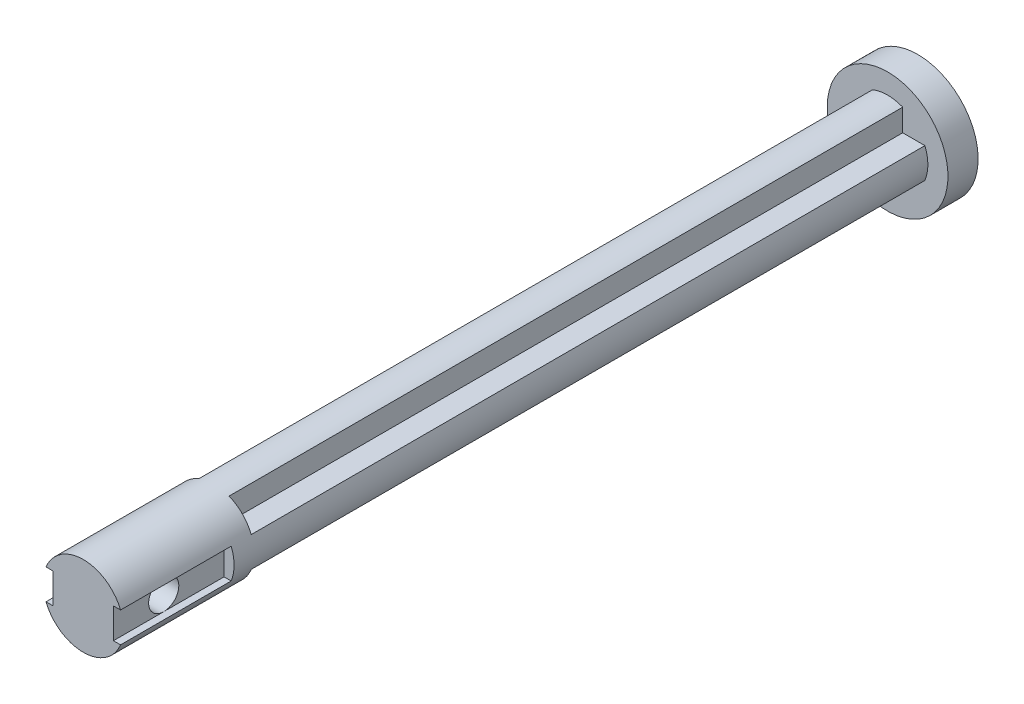
ISO-10303-21;
HEADER;
FILE_DESCRIPTION(('STEP AP214'),'2;1');
FILE_NAME('part.step','',(''),(''),'','','');
FILE_SCHEMA(('AUTOMOTIVE_DESIGN { 1 0 10303 214 1 1 1 1 }'));
ENDSEC;
DATA;
#1=APPLICATION_CONTEXT('core data for automotive mechanical design processes');
#2=APPLICATION_PROTOCOL_DEFINITION('international standard','automotive_design',2000,#1);
#3=PRODUCT_CONTEXT('',#1,'mechanical');
#4=PRODUCT('Part','Part','',(#3));
#5=PRODUCT_RELATED_PRODUCT_CATEGORY('part','',(#4));
#6=PRODUCT_DEFINITION_FORMATION('','',#4);
#7=PRODUCT_DEFINITION_CONTEXT('part definition',#1,'design');
#8=PRODUCT_DEFINITION('design','',#6,#7);
#9=PRODUCT_DEFINITION_SHAPE('','',#8);
#10=(LENGTH_UNIT() NAMED_UNIT(*) SI_UNIT(.MILLI.,.METRE.));
#11=(NAMED_UNIT(*) PLANE_ANGLE_UNIT() SI_UNIT($,.RADIAN.));
#12=(NAMED_UNIT(*) SI_UNIT($,.STERADIAN.) SOLID_ANGLE_UNIT());
#13=UNCERTAINTY_MEASURE_WITH_UNIT(LENGTH_MEASURE(1.E-05),#10,'distance_accuracy_value','');
#14=(GEOMETRIC_REPRESENTATION_CONTEXT(3) GLOBAL_UNCERTAINTY_ASSIGNED_CONTEXT((#13)) GLOBAL_UNIT_ASSIGNED_CONTEXT((#10,
#11,#12)) REPRESENTATION_CONTEXT('',''));
#15=CARTESIAN_POINT('',(0.,0.,0.));
#16=DIRECTION('',(0.,0.,1.));
#17=DIRECTION('',(1.,0.,0.));
#18=AXIS2_PLACEMENT_3D('',#15,#16,#17);
#19=CARTESIAN_POINT('',(3.,0.,69.));
#20=DIRECTION('',(-1.,0.,0.));
#21=DIRECTION('',(0.,0.,1.));
#22=AXIS2_PLACEMENT_3D('',#19,#20,#21);
#23=PLANE('',#22);
#24=CARTESIAN_POINT('',(3.,0.,75.));
#25=DIRECTION('',(1.,0.,0.));
#26=DIRECTION('',(0.,0.,-1.));
#27=AXIS2_PLACEMENT_3D('',#24,#25,#26);
#28=CIRCLE('',#27,1.5);
#29=CARTESIAN_POINT('',(3.,1.5,75.));
#30=VERTEX_POINT('',#29);
#31=CARTESIAN_POINT('',(3.,-1.5,75.));
#32=VERTEX_POINT('',#31);
#33=EDGE_CURVE('E54',#30,#32,#28,.T.);
#34=ORIENTED_EDGE('',*,*,#33,.F.);
#35=DIRECTION('',(0.,0.,1.));
#36=VECTOR('',#35,1.);
#37=CARTESIAN_POINT('',(3.,1.5,69.));
#38=LINE('',#37,#36);
#39=CARTESIAN_POINT('',(3.,1.5,80.));
#40=VERTEX_POINT('',#39);
#41=EDGE_CURVE('E381',#30,#40,#38,.T.);
#42=ORIENTED_EDGE('',*,*,#41,.T.);
#43=DIRECTION('',(0.,-1.,0.));
#44=VECTOR('',#43,1.);
#45=CARTESIAN_POINT('',(3.,0.,80.));
#46=LINE('',#45,#44);
#47=CARTESIAN_POINT('',(3.,-1.5,80.));
#48=VERTEX_POINT('',#47);
#49=EDGE_CURVE('E366',#40,#48,#46,.T.);
#50=ORIENTED_EDGE('',*,*,#49,.T.);
#51=DIRECTION('',(0.,0.,1.));
#52=VECTOR('',#51,1.);
#53=CARTESIAN_POINT('',(3.,-1.5,69.));
#54=LINE('',#53,#52);
#55=EDGE_CURVE('E364',#32,#48,#54,.T.);
#56=ORIENTED_EDGE('',*,*,#55,.F.);
#57=EDGE_LOOP('',(#34,#42,#50,#56));
#58=FACE_BOUND('',#57,.T.);
#59=ADVANCED_FACE('F41',(#58),#23,.F.);
#60=CARTESIAN_POINT('',(-3.,0.,69.));
#61=DIRECTION('',(-1.,0.,0.));
#62=DIRECTION('',(0.,-1.,0.));
#63=AXIS2_PLACEMENT_3D('',#60,#61,#62);
#64=PLANE('',#63);
#65=CARTESIAN_POINT('',(-3.,0.,75.));
#66=DIRECTION('',(-1.,0.,0.));
#67=DIRECTION('',(0.,-1.,0.));
#68=AXIS2_PLACEMENT_3D('',#65,#66,#67);
#69=CIRCLE('',#68,1.5);
#70=CARTESIAN_POINT('',(-3.,-1.5,75.));
#71=VERTEX_POINT('',#70);
#72=CARTESIAN_POINT('',(-3.,1.5,75.));
#73=VERTEX_POINT('',#72);
#74=EDGE_CURVE('E64',#71,#73,#69,.T.);
#75=ORIENTED_EDGE('',*,*,#74,.F.);
#76=DIRECTION('',(0.,0.,1.));
#77=VECTOR('',#76,1.);
#78=CARTESIAN_POINT('',(-3.,-1.5,69.));
#79=LINE('',#78,#77);
#80=CARTESIAN_POINT('',(-3.,-1.5,80.));
#81=VERTEX_POINT('',#80);
#82=EDGE_CURVE('E405',#71,#81,#79,.T.);
#83=ORIENTED_EDGE('',*,*,#82,.T.);
#84=DIRECTION('',(0.,-1.,0.));
#85=VECTOR('',#84,1.);
#86=CARTESIAN_POINT('',(-3.,0.,80.));
#87=LINE('',#86,#85);
#88=CARTESIAN_POINT('',(-3.,1.5,80.));
#89=VERTEX_POINT('',#88);
#90=EDGE_CURVE('E406',#89,#81,#87,.T.);
#91=ORIENTED_EDGE('',*,*,#90,.F.);
#92=DIRECTION('',(0.,0.,1.));
#93=VECTOR('',#92,1.);
#94=CARTESIAN_POINT('',(-3.,1.5,69.));
#95=LINE('',#94,#93);
#96=EDGE_CURVE('E407',#73,#89,#95,.T.);
#97=ORIENTED_EDGE('',*,*,#96,.F.);
#98=EDGE_LOOP('',(#75,#83,#91,#97));
#99=FACE_BOUND('',#98,.T.);
#100=ADVANCED_FACE('F334',(#99),#64,.T.);
#101=CARTESIAN_POINT('',(0.,0.,80.));
#102=DIRECTION('',(0.,0.,1.));
#103=DIRECTION('',(1.,0.,0.));
#104=AXIS2_PLACEMENT_3D('',#101,#102,#103);
#105=PLANE('',#104);
#106=CARTESIAN_POINT('',(0.,0.,80.));
#107=DIRECTION('',(0.,0.,1.));
#108=DIRECTION('',(1.,0.,0.));
#109=AXIS2_PLACEMENT_3D('',#106,#107,#108);
#110=CIRCLE('',#109,4.);
#111=CARTESIAN_POINT('',(3.70809924354783,1.5,80.));
#112=VERTEX_POINT('',#111);
#113=CARTESIAN_POINT('',(-3.70809924354783,1.5,80.));
#114=VERTEX_POINT('',#113);
#115=EDGE_CURVE('E207',#112,#114,#110,.T.);
#116=ORIENTED_EDGE('',*,*,#115,.T.);
#117=DIRECTION('',(1.,0.,0.));
#118=VECTOR('',#117,1.);
#119=CARTESIAN_POINT('',(0.,1.5,80.));
#120=LINE('',#119,#118);
#121=EDGE_CURVE('E382',#114,#89,#120,.T.);
#122=ORIENTED_EDGE('',*,*,#121,.T.);
#123=ORIENTED_EDGE('',*,*,#90,.T.);
#124=DIRECTION('',(1.,0.,0.));
#125=VECTOR('',#124,1.);
#126=CARTESIAN_POINT('',(0.,-1.5,80.));
#127=LINE('',#126,#125);
#128=CARTESIAN_POINT('',(-3.70809924354783,-1.5,80.));
#129=VERTEX_POINT('',#128);
#130=EDGE_CURVE('E415',#129,#81,#127,.T.);
#131=ORIENTED_EDGE('',*,*,#130,.F.);
#132=CARTESIAN_POINT('',(3.70809924354783,-1.5,80.));
#133=VERTEX_POINT('',#132);
#134=EDGE_CURVE('E215',#129,#133,#110,.T.);
#135=ORIENTED_EDGE('',*,*,#134,.T.);
#136=DIRECTION('',(1.,0.,0.));
#137=VECTOR('',#136,1.);
#138=CARTESIAN_POINT('',(0.,-1.5,80.));
#139=LINE('',#138,#137);
#140=EDGE_CURVE('E389',#48,#133,#139,.T.);
#141=ORIENTED_EDGE('',*,*,#140,.F.);
#142=ORIENTED_EDGE('',*,*,#49,.F.);
#143=DIRECTION('',(1.,0.,0.));
#144=VECTOR('',#143,1.);
#145=CARTESIAN_POINT('',(0.,1.5,80.));
#146=LINE('',#145,#144);
#147=EDGE_CURVE('E383',#40,#112,#146,.T.);
#148=ORIENTED_EDGE('',*,*,#147,.T.);
#149=EDGE_LOOP('',(#116,#122,#123,#131,#135,#141,#142,#148));
#150=FACE_BOUND('',#149,.T.);
#151=ADVANCED_FACE('F338',(#150),#105,.T.);
#152=CARTESIAN_POINT('',(0.,1.49999999999998,67.));
#153=DIRECTION('',(0.,1.,0.));
#154=DIRECTION('',(-1.,0.,0.));
#155=AXIS2_PLACEMENT_3D('',#152,#153,#154);
#156=PLANE('',#155);
#157=DIRECTION('',(1.,0.,0.));
#158=VECTOR('',#157,1.);
#159=CARTESIAN_POINT('',(0.,1.49999999999998,0.));
#160=LINE('',#159,#158);
#161=CARTESIAN_POINT('',(-3.70809924354783,1.5,0.));
#162=VERTEX_POINT('',#161);
#163=CARTESIAN_POINT('',(-1.50000000000001,1.49999999999999,0.));
#164=VERTEX_POINT('',#163);
#165=EDGE_CURVE('E191',#162,#164,#160,.T.);
#166=ORIENTED_EDGE('',*,*,#165,.F.);
#167=DIRECTION('',(0.,0.,-1.));
#168=VECTOR('',#167,1.);
#169=CARTESIAN_POINT('',(-3.70809924354783,1.5,67.));
#170=LINE('',#169,#168);
#171=CARTESIAN_POINT('',(-3.70809924354783,1.5,67.));
#172=VERTEX_POINT('',#171);
#173=EDGE_CURVE('E11',#172,#162,#170,.T.);
#174=ORIENTED_EDGE('',*,*,#173,.F.);
#175=DIRECTION('',(1.,0.,0.));
#176=VECTOR('',#175,1.);
#177=CARTESIAN_POINT('',(0.,1.49999999999998,67.));
#178=LINE('',#177,#176);
#179=CARTESIAN_POINT('',(-1.50000000000001,1.49999999999999,67.));
#180=VERTEX_POINT('',#179);
#181=EDGE_CURVE('E242',#172,#180,#178,.T.);
#182=ORIENTED_EDGE('',*,*,#181,.T.);
#183=DIRECTION('',(0.,0.,-1.));
#184=VECTOR('',#183,1.);
#185=CARTESIAN_POINT('',(-1.50000000000001,1.49999999999999,67.));
#186=LINE('',#185,#184);
#187=EDGE_CURVE('E210',#180,#164,#186,.T.);
#188=ORIENTED_EDGE('',*,*,#187,.T.);
#189=EDGE_LOOP('',(#166,#174,#182,#188));
#190=FACE_BOUND('',#189,.T.);
#191=ADVANCED_FACE('F43',(#190),#156,.T.);
#192=CARTESIAN_POINT('',(0.,-1.5,67.));
#193=DIRECTION('',(0.,1.,0.));
#194=DIRECTION('',(-1.,0.,0.));
#195=AXIS2_PLACEMENT_3D('',#192,#193,#194);
#196=PLANE('',#195);
#197=DIRECTION('',(1.,0.,0.));
#198=VECTOR('',#197,1.);
#199=CARTESIAN_POINT('',(0.,-1.5,0.));
#200=LINE('',#199,#198);
#201=CARTESIAN_POINT('',(-3.70809924354783,-1.5,0.));
#202=VERTEX_POINT('',#201);
#203=CARTESIAN_POINT('',(-1.50000000000003,-1.5,0.));
#204=VERTEX_POINT('',#203);
#205=EDGE_CURVE('E192',#202,#204,#200,.T.);
#206=ORIENTED_EDGE('',*,*,#205,.T.);
#207=DIRECTION('',(0.,0.,-1.));
#208=VECTOR('',#207,1.);
#209=CARTESIAN_POINT('',(-1.50000000000003,-1.5,67.));
#210=LINE('',#209,#208);
#211=CARTESIAN_POINT('',(-1.50000000000003,-1.5,67.));
#212=VERTEX_POINT('',#211);
#213=EDGE_CURVE('E270',#212,#204,#210,.T.);
#214=ORIENTED_EDGE('',*,*,#213,.F.);
#215=DIRECTION('',(1.,0.,0.));
#216=VECTOR('',#215,1.);
#217=CARTESIAN_POINT('',(0.,-1.5,67.));
#218=LINE('',#217,#216);
#219=CARTESIAN_POINT('',(-3.70809924354783,-1.5,67.));
#220=VERTEX_POINT('',#219);
#221=EDGE_CURVE('E272',#220,#212,#218,.T.);
#222=ORIENTED_EDGE('',*,*,#221,.F.);
#223=DIRECTION('',(0.,0.,-1.));
#224=VECTOR('',#223,1.);
#225=CARTESIAN_POINT('',(-3.70809924354783,-1.5,67.));
#226=LINE('',#225,#224);
#227=EDGE_CURVE('E47',#220,#202,#226,.T.);
#228=ORIENTED_EDGE('',*,*,#227,.T.);
#229=EDGE_LOOP('',(#206,#214,#222,#228));
#230=FACE_BOUND('',#229,.T.);
#231=ADVANCED_FACE('F271',(#230),#196,.F.);
#232=CARTESIAN_POINT('',(-1.50000000000002,0.,67.));
#233=DIRECTION('',(-1.,0.,0.));
#234=DIRECTION('',(0.,-1.,0.));
#235=AXIS2_PLACEMENT_3D('',#232,#233,#234);
#236=PLANE('',#235);
#237=DIRECTION('',(0.,1.,0.));
#238=VECTOR('',#237,1.);
#239=CARTESIAN_POINT('',(-1.50000000000002,0.,0.));
#240=LINE('',#239,#238);
#241=CARTESIAN_POINT('',(-1.50000000000005,-3.70809924354781,0.));
#242=VERTEX_POINT('',#241);
#243=EDGE_CURVE('E218',#242,#204,#240,.T.);
#244=ORIENTED_EDGE('',*,*,#243,.F.);
#245=DIRECTION('',(0.,0.,-1.));
#246=VECTOR('',#245,1.);
#247=CARTESIAN_POINT('',(-1.50000000000005,-3.70809924354781,67.));
#248=LINE('',#247,#246);
#249=CARTESIAN_POINT('',(-1.50000000000005,-3.70809924354781,67.));
#250=VERTEX_POINT('',#249);
#251=EDGE_CURVE('E262',#250,#242,#248,.T.);
#252=ORIENTED_EDGE('',*,*,#251,.F.);
#253=DIRECTION('',(0.,1.,0.));
#254=VECTOR('',#253,1.);
#255=CARTESIAN_POINT('',(-1.50000000000002,0.,67.));
#256=LINE('',#255,#254);
#257=EDGE_CURVE('E287',#250,#212,#256,.T.);
#258=ORIENTED_EDGE('',*,*,#257,.T.);
#259=ORIENTED_EDGE('',*,*,#213,.T.);
#260=EDGE_LOOP('',(#244,#252,#258,#259));
#261=FACE_BOUND('',#260,.T.);
#262=ADVANCED_FACE('F512',(#261),#236,.T.);
#263=CARTESIAN_POINT('',(1.49999999999998,0.,67.));
#264=DIRECTION('',(-1.,0.,0.));
#265=DIRECTION('',(0.,-1.,0.));
#266=AXIS2_PLACEMENT_3D('',#263,#264,#265);
#267=PLANE('',#266);
#268=DIRECTION('',(0.,1.,0.));
#269=VECTOR('',#268,1.);
#270=CARTESIAN_POINT('',(1.49999999999998,0.,0.));
#271=LINE('',#270,#269);
#272=CARTESIAN_POINT('',(1.49999999999995,-3.70809924354785,0.));
#273=VERTEX_POINT('',#272);
#274=CARTESIAN_POINT('',(1.49999999999997,-1.5,0.));
#275=VERTEX_POINT('',#274);
#276=EDGE_CURVE('E221',#273,#275,#271,.T.);
#277=ORIENTED_EDGE('',*,*,#276,.T.);
#278=DIRECTION('',(0.,0.,-1.));
#279=VECTOR('',#278,1.);
#280=CARTESIAN_POINT('',(1.49999999999997,-1.5,67.));
#281=LINE('',#280,#279);
#282=CARTESIAN_POINT('',(1.49999999999997,-1.5,67.));
#283=VERTEX_POINT('',#282);
#284=EDGE_CURVE('E256',#283,#275,#281,.T.);
#285=ORIENTED_EDGE('',*,*,#284,.F.);
#286=DIRECTION('',(0.,1.,0.));
#287=VECTOR('',#286,1.);
#288=CARTESIAN_POINT('',(1.49999999999998,0.,67.));
#289=LINE('',#288,#287);
#290=CARTESIAN_POINT('',(1.49999999999995,-3.70809924354785,67.));
#291=VERTEX_POINT('',#290);
#292=EDGE_CURVE('E291',#291,#283,#289,.T.);
#293=ORIENTED_EDGE('',*,*,#292,.F.);
#294=DIRECTION('',(0.,0.,-1.));
#295=VECTOR('',#294,1.);
#296=CARTESIAN_POINT('',(1.49999999999995,-3.70809924354785,67.));
#297=LINE('',#296,#295);
#298=EDGE_CURVE('E261',#291,#273,#297,.T.);
#299=ORIENTED_EDGE('',*,*,#298,.T.);
#300=EDGE_LOOP('',(#277,#285,#293,#299));
#301=FACE_BOUND('',#300,.T.);
#302=ADVANCED_FACE('F520',(#301),#267,.F.);
#303=CARTESIAN_POINT('',(0.,-1.5,67.));
#304=DIRECTION('',(0.,-1.,0.));
#305=DIRECTION('',(1.,0.,0.));
#306=AXIS2_PLACEMENT_3D('',#303,#304,#305);
#307=PLANE('',#306);
#308=DIRECTION('',(-1.,0.,0.));
#309=VECTOR('',#308,1.);
#310=CARTESIAN_POINT('',(0.,-1.5,0.));
#311=LINE('',#310,#309);
#312=CARTESIAN_POINT('',(3.70809924354783,-1.5,0.));
#313=VERTEX_POINT('',#312);
#314=EDGE_CURVE('E229',#313,#275,#311,.T.);
#315=ORIENTED_EDGE('',*,*,#314,.F.);
#316=DIRECTION('',(0.,0.,-1.));
#317=VECTOR('',#316,1.);
#318=CARTESIAN_POINT('',(3.70809924354783,-1.5,67.));
#319=LINE('',#318,#317);
#320=CARTESIAN_POINT('',(3.70809924354783,-1.5,67.));
#321=VERTEX_POINT('',#320);
#322=EDGE_CURVE('E254',#321,#313,#319,.T.);
#323=ORIENTED_EDGE('',*,*,#322,.F.);
#324=DIRECTION('',(-1.,0.,0.));
#325=VECTOR('',#324,1.);
#326=CARTESIAN_POINT('',(0.,-1.5,67.));
#327=LINE('',#326,#325);
#328=EDGE_CURVE('E297',#321,#283,#327,.T.);
#329=ORIENTED_EDGE('',*,*,#328,.T.);
#330=ORIENTED_EDGE('',*,*,#284,.T.);
#331=EDGE_LOOP('',(#315,#323,#329,#330));
#332=FACE_BOUND('',#331,.T.);
#333=ADVANCED_FACE('F527',(#332),#307,.T.);
#334=CARTESIAN_POINT('',(0.,1.49999999999998,67.));
#335=DIRECTION('',(0.,-1.,0.));
#336=DIRECTION('',(1.,0.,0.));
#337=AXIS2_PLACEMENT_3D('',#334,#335,#336);
#338=PLANE('',#337);
#339=DIRECTION('',(-1.,0.,0.));
#340=VECTOR('',#339,1.);
#341=CARTESIAN_POINT('',(0.,1.49999999999998,0.));
#342=LINE('',#341,#340);
#343=CARTESIAN_POINT('',(3.70809924354785,1.49999999999996,0.));
#344=VERTEX_POINT('',#343);
#345=CARTESIAN_POINT('',(1.49999999999999,1.49999999999997,0.));
#346=VERTEX_POINT('',#345);
#347=EDGE_CURVE('E231',#344,#346,#342,.T.);
#348=ORIENTED_EDGE('',*,*,#347,.T.);
#349=DIRECTION('',(0.,0.,-1.));
#350=VECTOR('',#349,1.);
#351=CARTESIAN_POINT('',(1.49999999999999,1.49999999999997,67.));
#352=LINE('',#351,#350);
#353=CARTESIAN_POINT('',(1.49999999999999,1.49999999999997,67.));
#354=VERTEX_POINT('',#353);
#355=EDGE_CURVE('E248',#354,#346,#352,.T.);
#356=ORIENTED_EDGE('',*,*,#355,.F.);
#357=DIRECTION('',(-1.,0.,0.));
#358=VECTOR('',#357,1.);
#359=CARTESIAN_POINT('',(0.,1.49999999999998,67.));
#360=LINE('',#359,#358);
#361=CARTESIAN_POINT('',(3.70809924354785,1.49999999999996,67.));
#362=VERTEX_POINT('',#361);
#363=EDGE_CURVE('E296',#362,#354,#360,.T.);
#364=ORIENTED_EDGE('',*,*,#363,.F.);
#365=DIRECTION('',(0.,0.,-1.));
#366=VECTOR('',#365,1.);
#367=CARTESIAN_POINT('',(3.70809924354785,1.49999999999996,67.));
#368=LINE('',#367,#366);
#369=EDGE_CURVE('E252',#362,#344,#368,.T.);
#370=ORIENTED_EDGE('',*,*,#369,.T.);
#371=EDGE_LOOP('',(#348,#356,#364,#370));
#372=FACE_BOUND('',#371,.T.);
#373=ADVANCED_FACE('F320',(#372),#338,.F.);
#374=CARTESIAN_POINT('',(1.49999999999998,0.,67.));
#375=DIRECTION('',(1.,0.,0.));
#376=DIRECTION('',(0.,1.,0.));
#377=AXIS2_PLACEMENT_3D('',#374,#375,#376);
#378=PLANE('',#377);
#379=DIRECTION('',(0.,-1.,0.));
#380=VECTOR('',#379,1.);
#381=CARTESIAN_POINT('',(1.49999999999998,0.,0.));
#382=LINE('',#381,#380);
#383=CARTESIAN_POINT('',(1.50000000000001,3.70809924354783,0.));
#384=VERTEX_POINT('',#383);
#385=EDGE_CURVE('E232',#384,#346,#382,.T.);
#386=ORIENTED_EDGE('',*,*,#385,.F.);
#387=DIRECTION('',(0.,0.,-1.));
#388=VECTOR('',#387,1.);
#389=CARTESIAN_POINT('',(1.50000000000001,3.70809924354783,67.));
#390=LINE('',#389,#388);
#391=CARTESIAN_POINT('',(1.50000000000001,3.70809924354783,67.));
#392=VERTEX_POINT('',#391);
#393=EDGE_CURVE('E249',#392,#384,#390,.T.);
#394=ORIENTED_EDGE('',*,*,#393,.F.);
#395=DIRECTION('',(0.,-1.,0.));
#396=VECTOR('',#395,1.);
#397=CARTESIAN_POINT('',(1.49999999999998,0.,67.));
#398=LINE('',#397,#396);
#399=EDGE_CURVE('E304',#392,#354,#398,.T.);
#400=ORIENTED_EDGE('',*,*,#399,.T.);
#401=ORIENTED_EDGE('',*,*,#355,.T.);
#402=EDGE_LOOP('',(#386,#394,#400,#401));
#403=FACE_BOUND('',#402,.T.);
#404=ADVANCED_FACE('F311',(#403),#378,.T.);
#405=CARTESIAN_POINT('',(0.,0.,67.));
#406=DIRECTION('',(0.,0.,-1.));
#407=DIRECTION('',(-1.,0.,0.));
#408=AXIS2_PLACEMENT_3D('',#405,#406,#407);
#409=CYLINDRICAL_SURFACE('',#408,4.);
#410=CARTESIAN_POINT('',(0.,0.,69.));
#411=DIRECTION('',(0.,0.,1.));
#412=DIRECTION('',(1.,0.,0.));
#413=AXIS2_PLACEMENT_3D('',#410,#411,#412);
#414=CIRCLE('',#413,4.);
#415=CARTESIAN_POINT('',(-3.70809924354783,1.5,69.));
#416=VERTEX_POINT('',#415);
#417=CARTESIAN_POINT('',(-3.70809924354783,-1.5,69.));
#418=VERTEX_POINT('',#417);
#419=EDGE_CURVE('E425',#416,#418,#414,.T.);
#420=ORIENTED_EDGE('',*,*,#419,.F.);
#421=DIRECTION('',(0.,0.,1.));
#422=VECTOR('',#421,1.);
#423=CARTESIAN_POINT('',(-3.70809924354783,1.5,69.));
#424=LINE('',#423,#422);
#425=EDGE_CURVE('E396',#416,#114,#424,.T.);
#426=ORIENTED_EDGE('',*,*,#425,.T.);
#427=ORIENTED_EDGE('',*,*,#115,.F.);
#428=DIRECTION('',(0.,0.,1.));
#429=VECTOR('',#428,1.);
#430=CARTESIAN_POINT('',(3.70809924354783,1.5,69.));
#431=LINE('',#430,#429);
#432=CARTESIAN_POINT('',(3.70809924354783,1.5,69.));
#433=VERTEX_POINT('',#432);
#434=EDGE_CURVE('E380',#433,#112,#431,.T.);
#435=ORIENTED_EDGE('',*,*,#434,.F.);
#436=CARTESIAN_POINT('',(0.,0.,69.));
#437=DIRECTION('',(0.,0.,1.));
#438=DIRECTION('',(1.,0.,0.));
#439=AXIS2_PLACEMENT_3D('',#436,#437,#438);
#440=CIRCLE('',#439,4.);
#441=CARTESIAN_POINT('',(3.70809924354783,-1.5,69.));
#442=VERTEX_POINT('',#441);
#443=EDGE_CURVE('E394',#442,#433,#440,.T.);
#444=ORIENTED_EDGE('',*,*,#443,.F.);
#445=DIRECTION('',(0.,0.,1.));
#446=VECTOR('',#445,1.);
#447=CARTESIAN_POINT('',(3.70809924354783,-1.5,69.));
#448=LINE('',#447,#446);
#449=EDGE_CURVE('E374',#442,#133,#448,.T.);
#450=ORIENTED_EDGE('',*,*,#449,.T.);
#451=ORIENTED_EDGE('',*,*,#134,.F.);
#452=DIRECTION('',(0.,0.,1.));
#453=VECTOR('',#452,1.);
#454=CARTESIAN_POINT('',(-3.70809924354783,-1.5,69.));
#455=LINE('',#454,#453);
#456=EDGE_CURVE('E398',#418,#129,#455,.T.);
#457=ORIENTED_EDGE('',*,*,#456,.F.);
#458=EDGE_LOOP('',(#420,#426,#427,#435,#444,#450,#451,#457));
#459=FACE_BOUND('',#458,.T.);
#460=CARTESIAN_POINT('',(0.,0.,0.));
#461=DIRECTION('',(0.,0.,1.));
#462=DIRECTION('',(1.,0.,0.));
#463=AXIS2_PLACEMENT_3D('',#460,#461,#462);
#464=CIRCLE('',#463,4.);
#465=CARTESIAN_POINT('',(-1.49999999999999,3.70809924354784,0.));
#466=VERTEX_POINT('',#465);
#467=EDGE_CURVE('E240',#384,#466,#464,.T.);
#468=ORIENTED_EDGE('',*,*,#467,.T.);
#469=DIRECTION('',(0.,0.,-1.));
#470=VECTOR('',#469,1.);
#471=CARTESIAN_POINT('',(-1.49999999999999,3.70809924354784,67.));
#472=LINE('',#471,#470);
#473=CARTESIAN_POINT('',(-1.49999999999999,3.70809924354784,67.));
#474=VERTEX_POINT('',#473);
#475=EDGE_CURVE('E245',#474,#466,#472,.T.);
#476=ORIENTED_EDGE('',*,*,#475,.F.);
#477=CARTESIAN_POINT('',(0.,0.,67.));
#478=DIRECTION('',(0.,0.,1.));
#479=DIRECTION('',(1.,0.,0.));
#480=AXIS2_PLACEMENT_3D('',#477,#478,#479);
#481=CIRCLE('',#480,4.);
#482=EDGE_CURVE('E201',#474,#172,#481,.T.);
#483=ORIENTED_EDGE('',*,*,#482,.T.);
#484=ORIENTED_EDGE('',*,*,#173,.T.);
#485=CARTESIAN_POINT('',(0.,0.,0.));
#486=DIRECTION('',(0.,0.,1.));
#487=DIRECTION('',(1.,0.,0.));
#488=AXIS2_PLACEMENT_3D('',#485,#486,#487);
#489=CIRCLE('',#488,4.);
#490=EDGE_CURVE('E186',#162,#202,#489,.T.);
#491=ORIENTED_EDGE('',*,*,#490,.T.);
#492=ORIENTED_EDGE('',*,*,#227,.F.);
#493=EDGE_CURVE('E277',#220,#250,#481,.T.);
#494=ORIENTED_EDGE('',*,*,#493,.T.);
#495=ORIENTED_EDGE('',*,*,#251,.T.);
#496=CARTESIAN_POINT('',(0.,0.,0.));
#497=DIRECTION('',(0.,0.,1.));
#498=DIRECTION('',(1.,0.,0.));
#499=AXIS2_PLACEMENT_3D('',#496,#497,#498);
#500=CIRCLE('',#499,4.);
#501=EDGE_CURVE('E222',#242,#273,#500,.T.);
#502=ORIENTED_EDGE('',*,*,#501,.T.);
#503=ORIENTED_EDGE('',*,*,#298,.F.);
#504=EDGE_CURVE('E278',#291,#321,#481,.T.);
#505=ORIENTED_EDGE('',*,*,#504,.T.);
#506=ORIENTED_EDGE('',*,*,#322,.T.);
#507=CARTESIAN_POINT('',(0.,0.,0.));
#508=DIRECTION('',(0.,0.,1.));
#509=DIRECTION('',(1.,0.,0.));
#510=AXIS2_PLACEMENT_3D('',#507,#508,#509);
#511=CIRCLE('',#510,4.);
#512=EDGE_CURVE('E226',#313,#344,#511,.T.);
#513=ORIENTED_EDGE('',*,*,#512,.T.);
#514=ORIENTED_EDGE('',*,*,#369,.F.);
#515=EDGE_CURVE('E284',#362,#392,#481,.T.);
#516=ORIENTED_EDGE('',*,*,#515,.T.);
#517=ORIENTED_EDGE('',*,*,#393,.T.);
#518=EDGE_LOOP('',(#468,#476,#483,#484,#491,#492,#494,#495,#502,#503,#505,#506,#513,#514,#516,#517));
#519=FACE_BOUND('',#518,.T.);
#520=ADVANCED_FACE('F203',(#459,#519),#409,.T.);
#521=CARTESIAN_POINT('',(-1.50000000000002,0.,67.));
#522=DIRECTION('',(1.,0.,0.));
#523=DIRECTION('',(0.,1.,0.));
#524=AXIS2_PLACEMENT_3D('',#521,#522,#523);
#525=PLANE('',#524);
#526=DIRECTION('',(0.,-1.,0.));
#527=VECTOR('',#526,1.);
#528=CARTESIAN_POINT('',(-1.50000000000002,0.,0.));
#529=LINE('',#528,#527);
#530=EDGE_CURVE('E239',#466,#164,#529,.T.);
#531=ORIENTED_EDGE('',*,*,#530,.T.);
#532=ORIENTED_EDGE('',*,*,#187,.F.);
#533=DIRECTION('',(0.,-1.,0.));
#534=VECTOR('',#533,1.);
#535=CARTESIAN_POINT('',(-1.50000000000002,0.,67.));
#536=LINE('',#535,#534);
#537=EDGE_CURVE('E214',#474,#180,#536,.T.);
#538=ORIENTED_EDGE('',*,*,#537,.F.);
#539=ORIENTED_EDGE('',*,*,#475,.T.);
#540=EDGE_LOOP('',(#531,#532,#538,#539));
#541=FACE_BOUND('',#540,.T.);
#542=ADVANCED_FACE('F309',(#541),#525,.F.);
#543=CARTESIAN_POINT('',(0.,0.,67.));
#544=DIRECTION('',(0.,0.,1.));
#545=DIRECTION('',(1.,0.,0.));
#546=AXIS2_PLACEMENT_3D('',#543,#544,#545);
#547=PLANE('',#546);
#548=ORIENTED_EDGE('',*,*,#493,.F.);
#549=ORIENTED_EDGE('',*,*,#221,.T.);
#550=ORIENTED_EDGE('',*,*,#257,.F.);
#551=EDGE_LOOP('',(#548,#549,#550));
#552=FACE_BOUND('',#551,.T.);
#553=ADVANCED_FACE('F327',(#552),#547,.F.);
#554=ORIENTED_EDGE('',*,*,#504,.F.);
#555=ORIENTED_EDGE('',*,*,#292,.T.);
#556=ORIENTED_EDGE('',*,*,#328,.F.);
#557=EDGE_LOOP('',(#554,#555,#556));
#558=FACE_BOUND('',#557,.T.);
#559=ADVANCED_FACE('F321',(#558),#547,.F.);
#560=ORIENTED_EDGE('',*,*,#515,.F.);
#561=ORIENTED_EDGE('',*,*,#363,.T.);
#562=ORIENTED_EDGE('',*,*,#399,.F.);
#563=EDGE_LOOP('',(#560,#561,#562));
#564=FACE_BOUND('',#563,.T.);
#565=ADVANCED_FACE('F317',(#564),#547,.F.);
#566=ORIENTED_EDGE('',*,*,#181,.F.);
#567=ORIENTED_EDGE('',*,*,#482,.F.);
#568=ORIENTED_EDGE('',*,*,#537,.T.);
#569=EDGE_LOOP('',(#566,#567,#568));
#570=FACE_BOUND('',#569,.T.);
#571=ADVANCED_FACE('F306',(#570),#547,.F.);
#572=EDGE_CURVE('E353',#32,#30,#28,.T.);
#573=ORIENTED_EDGE('',*,*,#572,.F.);
#574=CARTESIAN_POINT('',(3.,-1.5,69.));
#575=VERTEX_POINT('',#574);
#576=EDGE_CURVE('E358',#575,#32,#54,.T.);
#577=ORIENTED_EDGE('',*,*,#576,.F.);
#578=DIRECTION('',(0.,-1.,0.));
#579=VECTOR('',#578,1.);
#580=CARTESIAN_POINT('',(3.,0.,69.));
#581=LINE('',#580,#579);
#582=CARTESIAN_POINT('',(3.,1.5,69.));
#583=VERTEX_POINT('',#582);
#584=EDGE_CURVE('E390',#583,#575,#581,.T.);
#585=ORIENTED_EDGE('',*,*,#584,.F.);
#586=EDGE_CURVE('E363',#583,#30,#38,.T.);
#587=ORIENTED_EDGE('',*,*,#586,.T.);
#588=EDGE_LOOP('',(#573,#577,#585,#587));
#589=FACE_BOUND('',#588,.T.);
#590=ADVANCED_FACE('F330',(#589),#23,.F.);
#591=CARTESIAN_POINT('',(0.,1.5,69.));
#592=DIRECTION('',(0.,-1.,0.));
#593=DIRECTION('',(1.,0.,0.));
#594=AXIS2_PLACEMENT_3D('',#591,#592,#593);
#595=PLANE('',#594);
#596=ORIENTED_EDGE('',*,*,#147,.F.);
#597=ORIENTED_EDGE('',*,*,#41,.F.);
#598=ORIENTED_EDGE('',*,*,#586,.F.);
#599=DIRECTION('',(1.,0.,0.));
#600=VECTOR('',#599,1.);
#601=CARTESIAN_POINT('',(0.,1.5,69.));
#602=LINE('',#601,#600);
#603=EDGE_CURVE('E371',#583,#433,#602,.T.);
#604=ORIENTED_EDGE('',*,*,#603,.T.);
#605=ORIENTED_EDGE('',*,*,#434,.T.);
#606=EDGE_LOOP('',(#596,#597,#598,#604,#605));
#607=FACE_BOUND('',#606,.T.);
#608=ADVANCED_FACE('F347',(#607),#595,.T.);
#609=CARTESIAN_POINT('',(0.,-1.5,69.));
#610=DIRECTION('',(0.,-1.,0.));
#611=DIRECTION('',(0.,0.,-1.));
#612=AXIS2_PLACEMENT_3D('',#609,#610,#611);
#613=PLANE('',#612);
#614=ORIENTED_EDGE('',*,*,#140,.T.);
#615=ORIENTED_EDGE('',*,*,#449,.F.);
#616=DIRECTION('',(1.,0.,0.));
#617=VECTOR('',#616,1.);
#618=CARTESIAN_POINT('',(0.,-1.5,69.));
#619=LINE('',#618,#617);
#620=EDGE_CURVE('E373',#575,#442,#619,.T.);
#621=ORIENTED_EDGE('',*,*,#620,.F.);
#622=ORIENTED_EDGE('',*,*,#576,.T.);
#623=ORIENTED_EDGE('',*,*,#55,.T.);
#624=EDGE_LOOP('',(#614,#615,#621,#622,#623));
#625=FACE_BOUND('',#624,.T.);
#626=ADVANCED_FACE('F352',(#625),#613,.F.);
#627=CARTESIAN_POINT('',(0.,0.,69.));
#628=DIRECTION('',(0.,0.,1.));
#629=DIRECTION('',(1.,0.,0.));
#630=AXIS2_PLACEMENT_3D('',#627,#628,#629);
#631=PLANE('',#630);
#632=ORIENTED_EDGE('',*,*,#584,.T.);
#633=ORIENTED_EDGE('',*,*,#620,.T.);
#634=ORIENTED_EDGE('',*,*,#443,.T.);
#635=ORIENTED_EDGE('',*,*,#603,.F.);
#636=EDGE_LOOP('',(#632,#633,#634,#635));
#637=FACE_BOUND('',#636,.T.);
#638=ADVANCED_FACE('F463',(#637),#631,.T.);
#639=CARTESIAN_POINT('',(0.,1.5,69.));
#640=DIRECTION('',(0.,-1.,0.));
#641=DIRECTION('',(1.,0.,0.));
#642=AXIS2_PLACEMENT_3D('',#639,#640,#641);
#643=PLANE('',#642);
#644=CARTESIAN_POINT('',(-3.,1.5,69.));
#645=VERTEX_POINT('',#644);
#646=EDGE_CURVE('E281',#645,#73,#95,.T.);
#647=ORIENTED_EDGE('',*,*,#646,.T.);
#648=ORIENTED_EDGE('',*,*,#96,.T.);
#649=ORIENTED_EDGE('',*,*,#121,.F.);
#650=ORIENTED_EDGE('',*,*,#425,.F.);
#651=DIRECTION('',(1.,0.,0.));
#652=VECTOR('',#651,1.);
#653=CARTESIAN_POINT('',(0.,1.5,69.));
#654=LINE('',#653,#652);
#655=EDGE_CURVE('E411',#416,#645,#654,.T.);
#656=ORIENTED_EDGE('',*,*,#655,.T.);
#657=EDGE_LOOP('',(#647,#648,#649,#650,#656));
#658=FACE_BOUND('',#657,.T.);
#659=ADVANCED_FACE('F456',(#658),#643,.T.);
#660=EDGE_CURVE('E430',#73,#71,#69,.T.);
#661=ORIENTED_EDGE('',*,*,#660,.F.);
#662=ORIENTED_EDGE('',*,*,#646,.F.);
#663=DIRECTION('',(0.,-1.,0.));
#664=VECTOR('',#663,1.);
#665=CARTESIAN_POINT('',(-3.,0.,69.));
#666=LINE('',#665,#664);
#667=CARTESIAN_POINT('',(-3.,-1.5,69.));
#668=VERTEX_POINT('',#667);
#669=EDGE_CURVE('E397',#645,#668,#666,.T.);
#670=ORIENTED_EDGE('',*,*,#669,.T.);
#671=EDGE_CURVE('E401',#668,#71,#79,.T.);
#672=ORIENTED_EDGE('',*,*,#671,.T.);
#673=EDGE_LOOP('',(#661,#662,#670,#672));
#674=FACE_BOUND('',#673,.T.);
#675=ADVANCED_FACE('F345',(#674),#64,.T.);
#676=CARTESIAN_POINT('',(0.,-1.5,69.));
#677=DIRECTION('',(0.,-1.,0.));
#678=DIRECTION('',(0.,0.,-1.));
#679=AXIS2_PLACEMENT_3D('',#676,#677,#678);
#680=PLANE('',#679);
#681=ORIENTED_EDGE('',*,*,#456,.T.);
#682=ORIENTED_EDGE('',*,*,#130,.T.);
#683=ORIENTED_EDGE('',*,*,#82,.F.);
#684=ORIENTED_EDGE('',*,*,#671,.F.);
#685=DIRECTION('',(1.,0.,0.));
#686=VECTOR('',#685,1.);
#687=CARTESIAN_POINT('',(0.,-1.5,69.));
#688=LINE('',#687,#686);
#689=EDGE_CURVE('E420',#418,#668,#688,.T.);
#690=ORIENTED_EDGE('',*,*,#689,.F.);
#691=EDGE_LOOP('',(#681,#682,#683,#684,#690));
#692=FACE_BOUND('',#691,.T.);
#693=ADVANCED_FACE('F453',(#692),#680,.F.);
#694=CARTESIAN_POINT('',(0.,0.,69.));
#695=DIRECTION('',(0.,0.,1.));
#696=DIRECTION('',(1.,0.,0.));
#697=AXIS2_PLACEMENT_3D('',#694,#695,#696);
#698=PLANE('',#697);
#699=ORIENTED_EDGE('',*,*,#655,.F.);
#700=ORIENTED_EDGE('',*,*,#419,.T.);
#701=ORIENTED_EDGE('',*,*,#689,.T.);
#702=ORIENTED_EDGE('',*,*,#669,.F.);
#703=EDGE_LOOP('',(#699,#700,#701,#702));
#704=FACE_BOUND('',#703,.T.);
#705=ADVANCED_FACE('F448',(#704),#698,.T.);
#706=CARTESIAN_POINT('',(-8.,0.,75.));
#707=DIRECTION('',(1.,0.,0.));
#708=DIRECTION('',(0.,0.,-1.));
#709=AXIS2_PLACEMENT_3D('',#706,#707,#708);
#710=CYLINDRICAL_SURFACE('',#709,1.5);
#711=ORIENTED_EDGE('',*,*,#74,.T.);
#712=ORIENTED_EDGE('',*,*,#660,.T.);
#713=EDGE_LOOP('',(#711,#712));
#714=FACE_BOUND('',#713,.T.);
#715=ORIENTED_EDGE('',*,*,#33,.T.);
#716=ORIENTED_EDGE('',*,*,#572,.T.);
#717=EDGE_LOOP('',(#715,#716));
#718=FACE_BOUND('',#717,.T.);
#719=ADVANCED_FACE('F441',(#714,#718),#710,.F.);
#720=CARTESIAN_POINT('',(0.,0.,0.));
#721=DIRECTION('',(0.,0.,-1.));
#722=DIRECTION('',(-1.,0.,0.));
#723=AXIS2_PLACEMENT_3D('',#720,#721,#722);
#724=PLANE('',#723);
#725=CARTESIAN_POINT('',(0.,0.,0.));
#726=DIRECTION('',(0.,0.,-1.));
#727=DIRECTION('',(-1.,0.,0.));
#728=AXIS2_PLACEMENT_3D('',#725,#726,#727);
#729=CIRCLE('',#728,6.);
#730=CARTESIAN_POINT('',(-6.,0.,0.));
#731=VERTEX_POINT('',#730);
#732=EDGE_CURVE('E427',#731,#731,#729,.T.);
#733=ORIENTED_EDGE('',*,*,#732,.F.);
#734=EDGE_LOOP('',(#733));
#735=FACE_BOUND('',#734,.T.);
#736=ORIENTED_EDGE('',*,*,#490,.F.);
#737=ORIENTED_EDGE('',*,*,#165,.T.);
#738=ORIENTED_EDGE('',*,*,#530,.F.);
#739=ORIENTED_EDGE('',*,*,#467,.F.);
#740=ORIENTED_EDGE('',*,*,#385,.T.);
#741=ORIENTED_EDGE('',*,*,#347,.F.);
#742=ORIENTED_EDGE('',*,*,#512,.F.);
#743=ORIENTED_EDGE('',*,*,#314,.T.);
#744=ORIENTED_EDGE('',*,*,#276,.F.);
#745=ORIENTED_EDGE('',*,*,#501,.F.);
#746=ORIENTED_EDGE('',*,*,#243,.T.);
#747=ORIENTED_EDGE('',*,*,#205,.F.);
#748=EDGE_LOOP('',(#736,#737,#738,#739,#740,#741,#742,#743,#744,#745,#746,#747));
#749=FACE_BOUND('',#748,.T.);
#750=ADVANCED_FACE('F188',(#735,#749),#724,.F.);
#751=CARTESIAN_POINT('',(0.,0.,-3.));
#752=DIRECTION('',(0.,0.,1.));
#753=DIRECTION('',(1.,0.,0.));
#754=AXIS2_PLACEMENT_3D('',#751,#752,#753);
#755=CYLINDRICAL_SURFACE('',#754,6.);
#756=CARTESIAN_POINT('',(0.,0.,-3.));
#757=DIRECTION('',(0.,0.,-1.));
#758=DIRECTION('',(-1.,0.,0.));
#759=AXIS2_PLACEMENT_3D('',#756,#757,#758);
#760=CIRCLE('',#759,6.);
#761=CARTESIAN_POINT('',(-6.,0.,-3.));
#762=VERTEX_POINT('',#761);
#763=EDGE_CURVE('E362',#762,#762,#760,.T.);
#764=ORIENTED_EDGE('',*,*,#763,.F.);
#765=EDGE_LOOP('',(#764));
#766=FACE_BOUND('',#765,.T.);
#767=ORIENTED_EDGE('',*,*,#732,.T.);
#768=EDGE_LOOP('',(#767));
#769=FACE_BOUND('',#768,.T.);
#770=ADVANCED_FACE('F440',(#766,#769),#755,.T.);
#771=CARTESIAN_POINT('',(0.,0.,-3.));
#772=DIRECTION('',(0.,0.,-1.));
#773=DIRECTION('',(-1.,0.,0.));
#774=AXIS2_PLACEMENT_3D('',#771,#772,#773);
#775=PLANE('',#774);
#776=ORIENTED_EDGE('',*,*,#763,.T.);
#777=EDGE_LOOP('',(#776));
#778=FACE_BOUND('',#777,.T.);
#779=ADVANCED_FACE('F434',(#778),#775,.T.);
#780=CLOSED_SHELL('',(#59,#100,#151,#191,#231,#262,#302,#333,#373,#404,#520,#542,#553,#559,#565,
#571,#590,#608,#626,#638,#659,#675,#693,#705,#719,#750,#770,#779));
#781=MANIFOLD_SOLID_BREP('B2',#780);
#782=ADVANCED_BREP_SHAPE_REPRESENTATION('',(#18,#781),#14);
#783=SHAPE_DEFINITION_REPRESENTATION(#9,#782);
ENDSEC;
END-ISO-10303-21;
